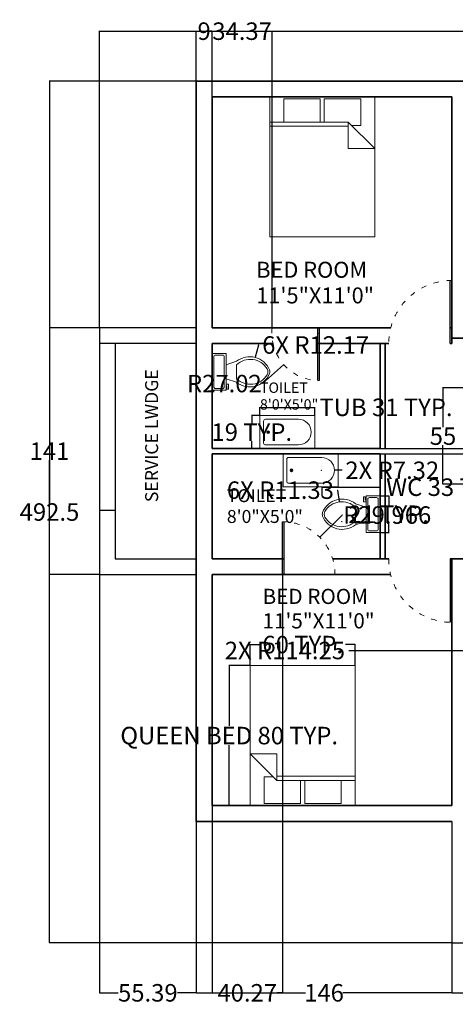
# Model space of a CAD drawing. Units: inches. Extents: x 37 to 687, y -399 to 163.
# Tile 1 of 4: x 37 to 286, y -399 to 163. Entities that reach past the tile are written whole.
import ezdxf

# ---------------------------------------------------------------- set-up
doc = ezdxf.new("R2010")
doc.units = ezdxf.units.IN
doc.header["$MEASUREMENT"] = 0
doc.linetypes.add('ACAD_ISO03W100', pattern=[30, 12, -18])
for name, color, linetype, lineweight in [('A-ANNO-DIMS', 2, 'Continuous', 18), ('A-AREA-IDEN', 7, 'Continuous', 18), ('A-DOOR', 4, 'Continuous', 25), ('A-DOOR-SWNG', 4, 'ACAD_ISO03W100', 13), ('A-FLOR-FIXT', 9, 'Continuous', 18), ('A-FLOR-OTLN', 7, 'Continuous', 25), ('A-FURN', 8, 'Continuous', 18), ('A-WALL', 7, 'Continuous', 35), ('A-WALL-OVHD', 7, 'ACAD_ISO03W100', 18)]:
    doc.layers.add(name, color=color, linetype=linetype, lineweight=lineweight)
doc.styles.get("Standard").update_dxf_attribs({"font": 'arial.ttf'})
doc.dimstyles.get("Standard").update_dxf_attribs({"dimtxt": 10, "dimasz": 0.18, "dimexe": 0.18, "dimexo": 0.0625, "dimgap": 0.09, "dimtad": 0, "dimtih": 1, "dimtoh": 1, "dimdec": 0, "dimzin": 0, "dimdsep": 46, "dimlunit": 3, "dimtxsty": 'Standard', "dimcen": 0.09, "dimadec": 0, "dimazin": 0, "dimtfac": 1, "dimtdec": 0, "dimtofl": 0, "dimtmove": 0, "dimatfit": 3, "dimfxl": 1, "dimtolj": 1, "dimtzin": 0, "dimarcsym": 0})

# ---------------------------------------------------------------- blocks, each defined once
blk = doc.blocks.new('Bed - Queen')
for p, q in [((0, -80.00003), (0, 0)), ((0, 0), (59.99999, 0)), ((59.99999, 0), (59.99999, -80.00003)), ((7.99999, -1.2), (28.79998, -1.2)), ((7.99999, -14.4), (7.99999, -1.2)), ((28.79998, -1.2), (28.79998, -14.4)), ((31.19999, -1.2), (51.99999, -1.2)), ((31.19999, -14.4), (31.19999, -1.2)), ((51.99999, -1.2), (51.99999, -16.4)), ((0, -14.4), (44.8, -14.4)), ((44.8, -16.8), (0, -16.8)), ((59.99999, -29.6), (44.8, -14.4)), ((44.8, -14.4), (44.8, -29.6)), ((51.99999, -16.4), (46.79936, -16.4)), ((44.8, -29.6), (59.99999, -29.6)), ((59.99999, -80.00003), (0, -80.00003))]:
    blk.add_line(p, q)
blk = doc.blocks.new('Toilet - top')
for p, q in [((9.5, -6), (9.5, -2)), ((-10, -8.5), (-8, -8.5)), ((-10, -9.5), (-10, -8.5)), ((-7, -9.5), (-10, -9.5)), ((-8, -8.5), (-8, -8)), ((-7, -8), (-7, -9.5)), ((-4, -8), (-6, -14)), ((4, -8), (6, -14)), ((4, -14), (-4, -14))]:
    blk.add_line(p, q)
blk.add_lwpolyline([(10.5, -8), (10.5, 0), (-10.5, 0), (-10.5, -8)], close=True)
for points in [[(-9.5, -2), (-9.5, -6)], [(8.5, -1), (-8.5, -1)], [(-8.5, -7), (8.5, -7)]]:
    blk.add_lwpolyline(points)
for centre, radius, start, end in [((-8.62, -1.88), 0.884, 81.8699, 188.1301), ((8.62, -1.88), 0.884, 351.8699, 98.1301), ((-8.62, -6.12), 0.884, 171.8699, 278.1301), ((8.62, -6.12), 0.884, 261.8699, 8.1301), ((3.52, -21.58), 12.17, 141.4691, 247.9714), ((4.2, -21.82), 11.33, 136.3677, 238.9468), ((-3.52, -21.58), 12.17, 292.0284, 38.5307), ((-4.2, -21.82), 11.33, 301.053, 43.6321), ((0, -27.88), 4, 245.7318, 294.2682), ((0, -29), 4, 254.8605, 285.1395)]:
    blk.add_arc(centre, radius, start, end)
blk = doc.blocks.new('Bath Tub - 26 x 60 in.')
for p, q in [((8, -18), (10, -18)), ((9, -17), (9, -19))]:
    blk.add_line(p, q)
blk.add_lwpolyline([(0, -36), (0, 0), (60, 0), (60, -36)], close=True)
for points in [[(4, -30), (4, -6)], [(6, -4), (42, -4)], [(42, -32), (6, -32)]]:
    blk.add_lwpolyline(points)
for radius in [1.5, 1]:
    blk.add_circle((9, -18), radius)
for centre, radius, start, end in [((5.75, -5.75), 1.77, 81.8699, 188.1301), ((42, -18), 14, 270, 90), ((5.75, -30.25), 1.77, 171.8699, 278.1301)]:
    blk.add_arc(centre, radius, start, end)
blk = doc.blocks.new('*D9')
at = {"layer": 'A-ANNO-DIMS', "color": 0, "lineweight": -2, "ltscale": 0.25, "transparency": 16777216}
for p, q in [((168.43, -205.68), (156.31, -205.68)), ((156.49, -205.86), (156.49, -240.12)), ((156.49, -285.5), (156.49, -251.25)), ((168.43, -285.68), (156.31, -285.68))]:
    blk.add_line(p, q, dxfattribs=at)
at = {"layer": 'A-ANNO-DIMS', "color": 0, "ltscale": 0.25, "transparency": 16777216}
for points in [[(156.46, -205.86), (156.52, -205.86), (156.49, -205.68)], [(156.46, -285.5), (156.52, -285.5), (156.49, -285.68)]]:
    blk.add_solid(points, dxfattribs=at)
at = {"layer": 'Defpoints', "color": 0, "ltscale": 0.25, "transparency": 16777216}
for p in [(168.49, -205.68), (156.49, -285.68), (168.49, -285.68)]:
    blk.add_point(p, dxfattribs=at)
at = {"layer": 'A-ANNO-DIMS', "color": 0, "ltscale": 0.25, "transparency": 16777216, "insert": (156.49, -245.68), "char_height": 10, "attachment_point": 5}
blk.add_mtext('\\A1;QUEEN BED 80 TYP.', dxfattribs=at)
blk = doc.blocks.new('*D10')
at = {"layer": 'A-ANNO-DIMS', "color": 0, "lineweight": -2, "ltscale": 0.25, "transparency": 16777216}
for p, q in [((168.49, -205.62), (168.49, -193.5)), ((168.67, -193.68), (174.04, -193.68)), ((228.31, -193.68), (222.95, -193.68)), ((228.49, -205.62), (228.49, -193.5))]:
    blk.add_line(p, q, dxfattribs=at)
at = {"layer": 'A-ANNO-DIMS', "color": 0, "ltscale": 0.25, "transparency": 16777216}
for points in [[(168.67, -193.65), (168.67, -193.71), (168.49, -193.68)], [(228.31, -193.65), (228.31, -193.71), (228.49, -193.68)]]:
    blk.add_solid(points, dxfattribs=at)
at = {"layer": 'Defpoints', "color": 0, "ltscale": 0.25, "transparency": 16777216}
for p in [(168.49, -193.68), (168.49, -205.68), (228.49, -205.68)]:
    blk.add_point(p, dxfattribs=at)
at = {"layer": 'A-ANNO-DIMS', "color": 0, "ltscale": 0.25, "transparency": 16777216, "insert": (198.49, -193.68), "char_height": 10, "attachment_point": 5}
blk.add_mtext('\\A1;60 TYP.', dxfattribs=at)
blk = doc.blocks.new('*D15')
at = {"layer": 'A-ANNO-DIMS', "color": 0, "lineweight": -2, "ltscale": 0.25, "transparency": 16777216}
for p, q in [((174.08, -62.8), (174.08, -57.97)), ((174.26, -58.15), (205.27, -58.15)), ((205.45, -62.8), (205.45, -57.97)), ((205.45, -58.15), (205.63, -58.15))]:
    blk.add_line(p, q, dxfattribs=at)
at = {"layer": 'A-ANNO-DIMS', "color": 0, "ltscale": 0.25, "transparency": 16777216}
for points in [[(174.26, -58.12), (174.26, -58.18), (174.08, -58.15)], [(205.27, -58.12), (205.27, -58.18), (205.45, -58.15)]]:
    blk.add_solid(points, dxfattribs=at)
at = {"layer": 'Defpoints', "color": 0, "ltscale": 0.25, "transparency": 16777216}
for p in [(205.45, -58.15), (174.08, -62.86), (205.45, -62.86)]:
    blk.add_point(p, dxfattribs=at)
at = {"layer": 'A-ANNO-DIMS', "color": 0, "ltscale": 0.25, "transparency": 16777216, "insert": (246.1, -58.15), "char_height": 10, "attachment_point": 5}
blk.add_mtext('\\A1;TUB 31 TYP.', dxfattribs=at)
blk = doc.blocks.new('*D16')
at = {"layer": 'A-ANNO-DIMS', "color": 0, "lineweight": -2, "ltscale": 0.25, "transparency": 16777216}
for p, q in [((174.02, -62.86), (169.2, -62.86)), ((169.38, -63.04), (169.38, -67.08)), ((169.38, -81.5), (169.38, -77.47)), ((174.02, -81.68), (169.2, -81.68))]:
    blk.add_line(p, q, dxfattribs=at)
at = {"layer": 'A-ANNO-DIMS', "color": 0, "ltscale": 0.25, "transparency": 16777216}
for points in [[(169.35, -63.04), (169.41, -63.04), (169.38, -62.86)], [(169.35, -81.5), (169.41, -81.5), (169.38, -81.68)]]:
    blk.add_solid(points, dxfattribs=at)
at = {"layer": 'Defpoints', "color": 0, "ltscale": 0.25, "transparency": 16777216}
for p in [(169.38, -62.86), (174.08, -62.86), (174.08, -81.68)]:
    blk.add_point(p, dxfattribs=at)
at = {"layer": 'A-ANNO-DIMS', "color": 0, "ltscale": 0.25, "transparency": 16777216, "insert": (169.38, -72.27), "char_height": 10, "attachment_point": 5}
blk.add_mtext('\\A1;19 TYP.', dxfattribs=at)
blk = doc.blocks.new('*D17')
at = {"layer": 'A-ANNO-DIMS', "color": 0, "lineweight": -2, "ltscale": 0.25, "transparency": 16777216}
for p, q in [((209.64, -108.64), (209.64, -103.57)), ((209.82, -103.75), (242.51, -103.75)), ((242.69, -108.64), (242.69, -103.57)), ((242.69, -103.75), (242.87, -103.75))]:
    blk.add_line(p, q, dxfattribs=at)
at = {"layer": 'A-ANNO-DIMS', "color": 0, "ltscale": 0.25, "transparency": 16777216}
for points in [[(209.82, -103.72), (209.82, -103.78), (209.64, -103.75)], [(242.51, -103.72), (242.51, -103.78), (242.69, -103.75)]]:
    blk.add_solid(points, dxfattribs=at)
at = {"layer": 'Defpoints', "color": 0, "ltscale": 0.25, "transparency": 16777216}
for p in [(242.69, -103.75), (209.64, -108.71), (242.69, -108.71)]:
    blk.add_point(p, dxfattribs=at)
at = {"layer": 'A-ANNO-DIMS', "color": 0, "ltscale": 0.25, "transparency": 16777216, "insert": (281.08, -103.75), "char_height": 10, "attachment_point": 5}
blk.add_mtext('\\A1;WC 33 TYP.', dxfattribs=at)
blk = doc.blocks.new('*D18')
at = {"layer": 'A-ANNO-DIMS', "color": 0, "lineweight": -2, "ltscale": 0.25, "transparency": 16777216}
for p, q in [((242.75, -108.71), (247.82, -108.71)), ((247.64, -108.89), (247.64, -114.09)), ((247.64, -129.53), (247.64, -124.32)), ((242.75, -129.71), (247.82, -129.71))]:
    blk.add_line(p, q, dxfattribs=at)
at = {"layer": 'A-ANNO-DIMS', "color": 0, "ltscale": 0.25, "transparency": 16777216}
for points in [[(247.61, -108.89), (247.67, -108.89), (247.64, -108.71)], [(247.61, -129.53), (247.67, -129.53), (247.64, -129.71)]]:
    blk.add_solid(points, dxfattribs=at)
at = {"layer": 'Defpoints', "color": 0, "ltscale": 0.25, "transparency": 16777216}
for p in [(242.69, -108.71), (242.69, -129.71), (247.64, -129.71)]:
    blk.add_point(p, dxfattribs=at)
at = {"layer": 'A-ANNO-DIMS', "color": 0, "ltscale": 0.25, "transparency": 16777216, "insert": (247.64, -119.21), "char_height": 10, "attachment_point": 5}
blk.add_mtext('\\A1;21 TYP.', dxfattribs=at)
blk = doc.blocks.new('*D22')
at = {"layer": 'A-ANNO-DIMS', "color": 0, "lineweight": -2, "ltscale": 0.25, "transparency": 16777216}
for p, q in [((292.25, -47.07), (278.48, -47.07)), ((278.66, -47.25), (278.66, -69.4)), ((278.66, -101.89), (278.66, -79.75)), ((292.25, -102.07), (278.48, -102.07))]:
    blk.add_line(p, q, dxfattribs=at)
at = {"layer": 'A-ANNO-DIMS', "color": 0, "ltscale": 0.25, "transparency": 16777216}
for points in [[(278.63, -47.25), (278.69, -47.25), (278.66, -47.07)], [(278.63, -101.89), (278.69, -101.89), (278.66, -102.07)]]:
    blk.add_solid(points, dxfattribs=at)
at = {"layer": 'Defpoints', "color": 0, "ltscale": 0.25, "transparency": 16777216}
for p in [(278.66, -47.07), (292.31, -47.07), (292.31, -102.07)]:
    blk.add_point(p, dxfattribs=at)
at = {"layer": 'A-ANNO-DIMS', "color": 0, "ltscale": 0.25, "transparency": 16777216, "insert": (278.66, -74.57), "char_height": 10, "attachment_point": 5}
blk.add_mtext('\\A1;55', dxfattribs=at)
blk = doc.blocks.new('*D27')
at = {"layer": 'A-ANNO-DIMS', "color": 0, "lineweight": -2, "ltscale": 0.25, "transparency": 16777216}
for p, q in [((82.29, -12.62), (82.29, 157)), ((82.47, 156.82), (344.98, 156.82)), ((641.3, 156.82), (378.8, 156.82)), ((641.48, 53.47), (641.48, 157))]:
    blk.add_line(p, q, dxfattribs=at)
at = {"layer": 'A-ANNO-DIMS', "color": 0, "ltscale": 0.25, "transparency": 16777216}
for points in [[(82.47, 156.85), (82.47, 156.79), (82.29, 156.82)], [(641.3, 156.85), (641.3, 156.79), (641.48, 156.82)]]:
    blk.add_solid(points, dxfattribs=at)
at = {"layer": 'Defpoints', "color": 0, "ltscale": 0.25, "transparency": 16777216}
for p in [(641.48, 156.82), (641.48, 53.4), (82.29, -12.68)]:
    blk.add_point(p, dxfattribs=at)
at = {"layer": 'A-ANNO-DIMS', "color": 0, "ltscale": 0.25, "transparency": 16777216, "insert": (361.89, 156.82), "char_height": 10, "attachment_point": 5}
blk.add_mtext('\\A1;559.2', dxfattribs=at)
blk = doc.blocks.new('*D28')
at = {"layer": 'A-ANNO-DIMS', "color": 0, "lineweight": -2, "ltscale": 0.25, "transparency": 16777216}
for p, q in [((137.62, 128.32), (53.61, 128.32)), ((53.79, 128.14), (53.79, -112.73)), ((53.79, -363.99), (53.79, -123.12)), ((283.62, -364.17), (53.61, -364.17))]:
    blk.add_line(p, q, dxfattribs=at)
at = {"layer": 'A-ANNO-DIMS', "color": 0, "ltscale": 0.25, "transparency": 16777216}
for points in [[(53.76, 128.14), (53.82, 128.14), (53.79, 128.32)], [(53.76, -363.99), (53.82, -363.99), (53.79, -364.17)]]:
    blk.add_solid(points, dxfattribs=at)
at = {"layer": 'Defpoints', "color": 0, "ltscale": 0.25, "transparency": 16777216}
for p in [(137.69, 128.32), (53.79, -364.17), (283.69, -364.17)]:
    blk.add_point(p, dxfattribs=at)
at = {"layer": 'A-ANNO-DIMS', "color": 0, "ltscale": 0.25, "transparency": 16777216, "insert": (53.79, -117.93), "char_height": 10, "attachment_point": 5}
blk.add_mtext('\\A1;492.5', dxfattribs=at)
blk = doc.blocks.new('*D29')
at = {"layer": 'A-ANNO-DIMS', "color": 0, "lineweight": -2, "ltscale": 0.25, "transparency": 16777216}
for p, q in [((82.29, -153.75), (82.29, -392.85)), ((137.69, -294.75), (137.69, -392.85)), ((82.47, -392.67), (93.02, -392.67)), ((137.51, -392.67), (126.96, -392.67))]:
    blk.add_line(p, q, dxfattribs=at)
at = {"layer": 'A-ANNO-DIMS', "color": 0, "ltscale": 0.25, "transparency": 16777216}
for points in [[(82.47, -392.64), (82.47, -392.7), (82.29, -392.67)], [(137.51, -392.64), (137.51, -392.7), (137.69, -392.67)]]:
    blk.add_solid(points, dxfattribs=at)
at = {"layer": 'Defpoints', "color": 0, "ltscale": 0.25, "transparency": 16777216}
for p in [(82.29, -153.68), (137.69, -294.68), (137.69, -392.67)]:
    blk.add_point(p, dxfattribs=at)
at = {"layer": 'A-ANNO-DIMS', "color": 0, "ltscale": 0.25, "transparency": 16777216, "insert": (109.99, -392.67), "char_height": 10, "attachment_point": 5}
blk.add_mtext('\\A1;55.39', dxfattribs=at)
blk = doc.blocks.new('*D30')
at = {"layer": 'A-ANNO-DIMS', "color": 0, "lineweight": -2, "ltscale": 0.25, "transparency": 16777216}
for p, q in [((137.69, -294.75), (137.69, -392.85)), ((283.69, -294.75), (283.69, -392.85)), ((137.87, -392.67), (200.02, -392.67)), ((283.51, -392.67), (221.35, -392.67))]:
    blk.add_line(p, q, dxfattribs=at)
at = {"layer": 'A-ANNO-DIMS', "color": 0, "ltscale": 0.25, "transparency": 16777216}
for points in [[(137.87, -392.64), (137.87, -392.7), (137.69, -392.67)], [(283.51, -392.64), (283.51, -392.7), (283.69, -392.67)]]:
    blk.add_solid(points, dxfattribs=at)
at = {"layer": 'Defpoints', "color": 0, "ltscale": 0.25, "transparency": 16777216}
for p in [(137.69, -294.68), (283.69, -294.68), (283.69, -392.67)]:
    blk.add_point(p, dxfattribs=at)
at = {"layer": 'A-ANNO-DIMS', "color": 0, "ltscale": 0.25, "transparency": 16777216, "insert": (210.69, -392.67), "char_height": 10, "attachment_point": 5}
blk.add_mtext('\\A1;146', dxfattribs=at)
blk = doc.blocks.new('*D31')
at = {"layer": 'A-ANNO-DIMS', "color": 0, "lineweight": -2, "ltscale": 0.25, "transparency": 16777216}
for p, q in [((283.69, -364.23), (283.69, -392.85)), ((444.69, -364.23), (444.69, -392.85)), ((283.87, -392.67), (354.48, -392.67)), ((444.51, -392.67), (373.89, -392.67))]:
    blk.add_line(p, q, dxfattribs=at)
at = {"layer": 'A-ANNO-DIMS', "color": 0, "ltscale": 0.25, "transparency": 16777216}
for points in [[(283.87, -392.64), (283.87, -392.7), (283.69, -392.67)], [(444.51, -392.64), (444.51, -392.7), (444.69, -392.67)]]:
    blk.add_solid(points, dxfattribs=at)
at = {"layer": 'Defpoints', "color": 0, "ltscale": 0.25, "transparency": 16777216}
for p in [(283.69, -364.17), (444.69, -364.17), (444.69, -392.67)]:
    blk.add_point(p, dxfattribs=at)
at = {"layer": 'A-ANNO-DIMS', "color": 0, "ltscale": 0.25, "transparency": 16777216, "insert": (364.19, -392.67), "char_height": 10, "attachment_point": 5}
blk.add_mtext('\\A1;161', dxfattribs=at)
blk = doc.blocks.new('*D40')
at = {"layer": 'A-ANNO-DIMS', "color": 0, "lineweight": -2, "ltscale": 0.25, "transparency": 16777216}
for p, q in [((82.23, -12.68), (53.61, -12.68)), ((53.79, -12.86), (53.79, -78.07)), ((53.79, -153.5), (53.79, -88.3)), ((82.23, -153.68), (53.61, -153.68))]:
    blk.add_line(p, q, dxfattribs=at)
at = {"layer": 'A-ANNO-DIMS', "color": 0, "ltscale": 0.25, "transparency": 16777216}
for points in [[(53.76, -12.86), (53.82, -12.86), (53.79, -12.68)], [(53.76, -153.5), (53.82, -153.5), (53.79, -153.68)]]:
    blk.add_solid(points, dxfattribs=at)
at = {"layer": 'Defpoints', "color": 0, "ltscale": 0.25, "transparency": 16777216}
for p in [(53.79, -12.68), (82.29, -12.68), (82.29, -153.68)]:
    blk.add_point(p, dxfattribs=at)
at = {"layer": 'A-ANNO-DIMS', "color": 0, "ltscale": 0.25, "transparency": 16777216, "insert": (53.79, -83.18), "char_height": 10, "attachment_point": 5}
blk.add_mtext('\\A1;141', dxfattribs=at)
blk = doc.blocks.new('*D41')
at = {"layer": 'A-ANNO-DIMS', "color": 0, "lineweight": -2, "ltscale": 0.25, "transparency": 16777216}
for p, q in [((137.69, -12.62), (137.69, 157)), ((137.87, 156.82), (138.81, 156.82)), ((146.51, 156.82), (145.56, 156.82)), ((146.69, -12.62), (146.69, 157))]:
    blk.add_line(p, q, dxfattribs=at)
at = {"layer": 'A-ANNO-DIMS', "color": 0, "ltscale": 0.25, "transparency": 16777216}
for points in [[(137.87, 156.85), (137.87, 156.79), (137.69, 156.82)], [(146.51, 156.85), (146.51, 156.79), (146.69, 156.82)]]:
    blk.add_solid(points, dxfattribs=at)
at = {"layer": 'Defpoints', "color": 0, "ltscale": 0.25, "transparency": 16777216}
for p in [(146.69, 156.82), (137.69, -12.68), (146.69, -12.68)]:
    blk.add_point(p, dxfattribs=at)
at = {"layer": 'A-ANNO-DIMS', "color": 0, "ltscale": 0.25, "transparency": 16777216, "insert": (142.19, 156.82), "char_height": 10, "attachment_point": 5}
blk.add_mtext('\\A1;9', dxfattribs=at)
blk = doc.blocks.new('*D42')
at = {"layer": 'A-ANNO-DIMS', "color": 0, "lineweight": -2, "ltscale": 0.25, "transparency": 16777216}
for p, q in [((146.505166, 156.815421), (146.325166, 156.815421)), ((146.685166, -12.622079), (146.685166, 156.995421)), ((181.054232, -12.622079), (181.054232, 156.995421)), ((181.234232, 156.815421), (181.414232, 156.815421))]:
    blk.add_line(p, q, dxfattribs=at)
at = {"layer": 'A-ANNO-DIMS', "color": 0, "ltscale": 0.25, "transparency": 16777216}
for points in [[(146.505166, 156.845421), (146.505166, 156.785421), (146.685166, 156.815421)], [(181.234232, 156.845421), (181.234232, 156.785421), (181.054232, 156.815421)]]:
    blk.add_solid(points, dxfattribs=at)
at = {"layer": 'Defpoints', "color": 0, "ltscale": 0.25, "transparency": 16777216}
for p in [(181.054232, 156.815421), (146.685166, -12.684579), (181.054232, -12.684579)]:
    blk.add_point(p, dxfattribs=at)
at = {"layer": 'A-ANNO-DIMS', "color": 0, "ltscale": 0.25, "transparency": 16777216, "insert": (163.869699, 156.815421), "char_height": 10, "attachment_point": 5}
blk.add_mtext('\\A1;34.37', dxfattribs=at)
blk = doc.blocks.new('*D43')
at = {"layer": 'A-ANNO-DIMS', "color": 0, "lineweight": -2, "ltscale": 0.25, "transparency": 16777216}
for p, q in [((146.69, -153.75), (146.69, -392.85)), ((186.95, -153.75), (186.95, -392.85)), ((146.87, -392.67), (149.65, -392.67)), ((186.77, -392.67), (183.98, -392.67))]:
    blk.add_line(p, q, dxfattribs=at)
at = {"layer": 'A-ANNO-DIMS', "color": 0, "ltscale": 0.25, "transparency": 16777216}
for points in [[(146.87, -392.64), (146.87, -392.7), (146.69, -392.67)], [(186.77, -392.64), (186.77, -392.7), (186.95, -392.67)]]:
    blk.add_solid(points, dxfattribs=at)
at = {"layer": 'Defpoints', "color": 0, "ltscale": 0.25, "transparency": 16777216}
for p in [(146.69, -153.68), (186.95, -153.68), (186.95, -392.67)]:
    blk.add_point(p, dxfattribs=at)
at = {"layer": 'A-ANNO-DIMS', "color": 0, "ltscale": 0.25, "transparency": 16777216, "insert": (166.82, -392.67), "char_height": 10, "attachment_point": 5}
blk.add_mtext('\\A1;40.27', dxfattribs=at)
blk = doc.blocks.new('*D44')
at = {"layer": 'A-ANNO-DIMS', "color": 0, "lineweight": -2, "ltscale": 0.25, "transparency": 16777216}
for p, q in [((242.75, -81.68), (670.18, -81.68)), ((670, -81.68), (670, -81.5)), ((670, -81.5), (670.18, -81.5)), ((670, -84.5), (670, -81.86)), ((242.75, -84.68), (670.18, -84.68))]:
    blk.add_line(p, q, dxfattribs=at)
at = {"layer": 'A-ANNO-DIMS', "color": 0, "ltscale": 0.25, "transparency": 16777216}
for points in [[(669.97, -81.86), (670.03, -81.86), (670, -81.68)], [(669.97, -84.5), (670.03, -84.5), (670, -84.68)]]:
    blk.add_solid(points, dxfattribs=at)
at = {"layer": 'Defpoints', "color": 0, "ltscale": 0.25, "transparency": 16777216}
for p in [(242.69, -81.68), (670, -81.68), (242.69, -84.68)]:
    blk.add_point(p, dxfattribs=at)
at = {"layer": 'A-ANNO-DIMS', "color": 0, "ltscale": 0.25, "transparency": 16777216, "insert": (673.54, -81.5), "char_height": 10, "attachment_point": 5}
blk.add_mtext('\\A1;3', dxfattribs=at)
blk = doc.blocks.new('*D51')
at = {"layer": 'A-ANNO-DIMS', "color": 0, "lineweight": -2, "ltscale": 0.25, "transparency": 16777216}
for p, q in [((220.99, -119.68), (208.35, -132.22)), ((221.17, -119.68), (220.99, -119.68)), ((186.86, -153.45), (187.04, -153.45)), ((186.95, -153.54), (186.95, -153.36))]:
    blk.add_line(p, q, dxfattribs=at)
at = {"layer": 'A-ANNO-DIMS', "color": 0, "ltscale": 0.25, "transparency": 16777216}
blk.add_solid([(208.33, -132.19), (208.37, -132.24), (208.22, -132.34)], dxfattribs=at)
at = {"layer": 'Defpoints', "color": 0, "ltscale": 0.25, "transparency": 16777216}
for p in [(208.22, -132.34), (186.95, -153.45)]:
    blk.add_point(p, dxfattribs=at)
at = {"layer": 'A-ANNO-DIMS', "color": 0, "ltscale": 0.25, "transparency": 16777216, "insert": (246.8, -119.68), "char_height": 10, "attachment_point": 5}
blk.add_mtext('\\A1;R29.966', dxfattribs=at)
blk = doc.blocks.new('*D52')
at = {"layer": 'A-ANNO-DIMS', "color": 0, "lineweight": -2, "ltscale": 0.25, "transparency": 16777216}
for p, q in [((207.8, -15.8), (207.98, -15.8)), ((207.89, -15.89), (207.89, -15.71)), ((175.61, -44.55), (187.58, -33.89)), ((175.43, -44.55), (175.61, -44.55))]:
    blk.add_line(p, q, dxfattribs=at)
at = {"layer": 'A-ANNO-DIMS', "color": 0, "ltscale": 0.25, "transparency": 16777216}
blk.add_solid([(187.56, -33.87), (187.6, -33.92), (187.71, -33.77)], dxfattribs=at)
at = {"layer": 'Defpoints', "color": 0, "ltscale": 0.25, "transparency": 16777216}
for p in [(207.89, -15.8), (187.71, -33.77)]:
    blk.add_point(p, dxfattribs=at)
at = {"layer": 'A-ANNO-DIMS', "color": 0, "ltscale": 0.25, "transparency": 16777216, "insert": (153.73, -44.55), "char_height": 10, "attachment_point": 5}
blk.add_mtext('\\A1;R27.02', dxfattribs=at)
blk = doc.blocks.new('*D55')
at = {"layer": 'A-ANNO-DIMS', "color": 0, "lineweight": -2, "ltscale": 0.25, "transparency": 16777216}
for p, q in [((224.82, -197.06), (293.19, -197.06)), ((407.53, -197.06), (407.71, -197.06)), ((407.62, -197.15), (407.62, -196.97))]:
    blk.add_line(p, q, dxfattribs=at)
at = {"layer": 'A-ANNO-DIMS', "color": 0, "ltscale": 0.25, "transparency": 16777216}
blk.add_solid([(293.19, -197.03), (293.19, -197.09), (293.37, -197.06)], dxfattribs=at)
at = {"layer": 'Defpoints', "color": 0, "ltscale": 0.25, "transparency": 16777216}
for p in [(293.37, -197.06), (407.62, -197.06)]:
    blk.add_point(p, dxfattribs=at)
at = {"layer": 'A-ANNO-DIMS', "color": 0, "ltscale": 0.25, "transparency": 16777216, "insert": (188.33, -197.06), "char_height": 10, "attachment_point": 5}
blk.add_mtext('\\A1;2X R114.25', dxfattribs=at)
blk = doc.blocks.new('*D58')
at = {"layer": 'A-ANNO-DIMS', "color": 0, "lineweight": -2, "ltscale": 0.25, "transparency": 16777216}
for p, q in [((173.21, -22.51), (171.4, -29.4)), ((173.39, -22.51), (173.21, -22.51)), ((168.18, -41.34), (168.36, -41.34)), ((168.27, -41.43), (168.27, -41.25))]:
    blk.add_line(p, q, dxfattribs=at)
at = {"layer": 'A-ANNO-DIMS', "color": 0, "ltscale": 0.25, "transparency": 16777216}
blk.add_solid([(171.37, -29.39), (171.43, -29.41), (171.36, -29.57)], dxfattribs=at)
at = {"layer": 'Defpoints', "color": 0, "ltscale": 0.25, "transparency": 16777216}
for p in [(171.36, -29.57), (168.27, -41.34)]:
    blk.add_point(p, dxfattribs=at)
at = {"layer": 'A-ANNO-DIMS', "color": 0, "ltscale": 0.25, "transparency": 16777216, "insert": (205.91, -22.51), "char_height": 10, "attachment_point": 5}
blk.add_mtext('\\A1;6X R12.17', dxfattribs=at)
blk = doc.blocks.new('*D59')
at = {"layer": 'A-ANNO-DIMS', "color": 0, "lineweight": -2, "ltscale": 0.25, "transparency": 16777216}
for p, q in [((218.27, -105.44), (218.45, -105.44)), ((218.45, -105.44), (219.33, -112)), ((220.78, -123.41), (220.96, -123.41)), ((220.87, -123.5), (220.87, -123.32))]:
    blk.add_line(p, q, dxfattribs=at)
at = {"layer": 'A-ANNO-DIMS', "color": 0, "ltscale": 0.25, "transparency": 16777216}
blk.add_solid([(219.36, -112), (219.3, -112), (219.36, -112.18)], dxfattribs=at)
at = {"layer": 'Defpoints', "color": 0, "ltscale": 0.25, "transparency": 16777216}
for p in [(219.36, -112.18), (220.87, -123.41)]:
    blk.add_point(p, dxfattribs=at)
at = {"layer": 'A-ANNO-DIMS', "color": 0, "ltscale": 0.25, "transparency": 16777216, "insert": (185.75, -105.44), "char_height": 10, "attachment_point": 5}
blk.add_mtext('\\A1;6X R11.33', dxfattribs=at)
blk = doc.blocks.new('*D60')
at = {"layer": 'A-ANNO-DIMS', "color": 0, "lineweight": -2, "ltscale": 0.25, "transparency": 16777216}
for p, q in [((209.24, -94.1), (209.42, -94.1)), ((209.33, -94.19), (209.33, -94.01)), ((221.04, -94.1), (216.83, -94.1))]:
    blk.add_line(p, q, dxfattribs=at)
at = {"layer": 'A-ANNO-DIMS', "color": 0, "ltscale": 0.25, "transparency": 16777216}
blk.add_solid([(216.83, -94.07), (216.83, -94.13), (216.65, -94.1)], dxfattribs=at)
at = {"layer": 'Defpoints', "color": 0, "ltscale": 0.25, "transparency": 16777216}
for p in [(209.33, -94.1), (216.65, -94.1)]:
    blk.add_point(p, dxfattribs=at)
at = {"layer": 'A-ANNO-DIMS', "color": 0, "ltscale": 0.25, "transparency": 16777216, "insert": (249.68, -94.1), "char_height": 10, "attachment_point": 5}
blk.add_mtext('\\A1;2X R7.32', dxfattribs=at)

msp = doc.modelspace()

# ---------------------------------------------------------------- linework, layer by layer
at = {"layer": 'A-DOOR'}
for p, q in [((282.6852, -21.6846), (282.6852, 14.3724)), ((283.6852, -21.6846), (283.6852, 14.3724)), ((207.8937, -12.6846), (177.9197, -12.6846)), ((177.9197, -12.6846), (181.0542, -12.6846)), ((206.8937, -12.6846), (206.8937, -42.824)), ((207.8937, -12.6846), (207.8937, -42.824)), ((283.6852, -21.6846), (282.6852, -21.6846))]:
    msp.add_line(p, q, dxfattribs=at)
at = {"layer": 'A-DOOR', "ltscale": 0.25}
for p, q in [((186.9515, -153.6846), (186.9515, -123.4817)), ((187.9515, -153.6846), (187.9515, -123.4817)), ((283.6852, -144.6846), (282.6852, -144.6846)), ((282.6852, -144.6846), (282.6852, -180.9603)), ((283.6852, -144.6846), (283.6852, -180.9603)), ((186.9515, -153.6846), (216.9162, -153.6846))]:
    msp.add_line(p, q, dxfattribs=at)
at = {"layer": 'A-DOOR-SWNG', "ltscale": 0.25}
for centre, radius, start, end in [((283.6852, -21.6277), 36, 90, 180.09058), ((207.8937, -15.8039), 27.0201, 173.370656, 270), ((186.9515, -153.4474), 29.9657, 359.546558, 90), ((283.6852, -144.9592), 36.001, 179.562888, 270)]:
    msp.add_arc(centre, radius, start, end, dxfattribs=at)
at = {"layer": 'A-FLOR-OTLN', "ltscale": 0.25}
for p, q in [((137.6852, -12.6846), (82.2949, -12.6846)), ((82.2949, -12.6846), (82.2949, -153.6846)), ((137.6852, -21.6846), (82.2949, -21.6846)), ((91.2949, -21.6846), (91.2949, -144.6846)), ((91.2949, -117.1166), (82.2949, -117.1166)), ((91.2949, -144.6846), (137.6852, -144.6846)), ((82.2949, -153.6846), (137.6852, -153.6846))]:
    msp.add_line(p, q, dxfattribs=at)
at = {"layer": 'A-FLOR-OTLN'}
for p, q in [((283.6852, -294.6846), (283.6852, -364.1681)), ((283.6852, -364.1681), (444.6852, -364.1681))]:
    msp.add_line(p, q, dxfattribs=at)
at = {"layer": 'A-WALL'}
for p, q in [((137.6852, 128.3154), (595.6852, 128.3154)), ((137.6852, 128.3154), (137.6852, -294.6846)), ((137.6852, 119.3154), (137.6852, -12.6846)), ((146.6852, 119.3154), (146.6852, -12.6846)), ((146.6852, 119.3154), (283.6852, 119.3154)), ((283.6852, 119.3154), (283.6852, -21.6846)), ((248.8136, -12.6846), (146.6852, -12.6846)), ((283.6852, -12.6846), (282.6852, -12.6846)), ((137.6852, -21.6846), (137.6852, -81.6846)), ((146.6852, -21.6846), (146.6852, -81.6846)), ((181.5213, -21.6846), (146.6852, -21.6846)), ((247.6852, -21.6846), (206.8937, -21.6846)), ((242.6852, -81.6846), (242.6852, -21.6846)), ((245.6852, -81.6846), (245.6852, -21.6846)), ((283.6852, -21.6846), (282.6852, -21.6846)), ((146.6852, -81.6846), (242.6852, -81.6846)), ((137.6852, -84.6846), (137.6852, -144.6846)), ((146.6852, -84.6846), (242.6852, -84.6846)), ((146.6852, -84.6846), (146.6852, -144.6846)), ((242.6852, -144.6846), (242.6852, -84.6846)), ((245.6852, -144.6846), (245.6852, -84.6846)), ((146.6852, -144.6846), (187.9515, -144.6846)), ((215.6073, -144.6846), (242.6852, -144.6846)), ((247.6852, -144.6846), (242.6852, -144.6846)), ((290.6852, -144.6846), (282.6852, -144.6846)), ((283.6852, -285.6846), (283.6852, -144.6846)), ((146.6852, -153.6846), (242.6852, -153.6846)), ((146.6852, -153.6846), (146.6852, -285.6846)), ((248.7575, -153.6846), (242.6852, -153.6846)), ((283.6852, -153.6846), (282.6852, -153.6846)), ((283.6852, -259.1681), (283.6852, -285.6846)), ((146.6852, -285.6846), (283.6852, -285.6846)), ((137.6852, -294.6846), (283.6852, -294.6846))]:
    msp.add_line(p, q, dxfattribs=at)
at = {"layer": 'A-WALL', "ltscale": 0.25}
msp.add_line((292.6852, -18.6846), (283.6852, -18.6846), dxfattribs=at)
at = {"layer": 'A-WALL-OVHD', "ltscale": 0.25}
msp.add_line((439.6852, -18.6846), (283.6852, -18.6846), dxfattribs=at)

# ---------------------------------------------------------------- block references
at = {"layer": 'A-FLOR-FIXT', "ltscale": 0.25}
for p, rotation in [((146.6852, -37.8245), 90), ((242.6852, -119.2072), 270.0000000000002)]:
    msp.add_blockref('Toilet - top', p, dxfattribs=dict(at, rotation=rotation))
at = {"layer": 'A-FLOR-FIXT', "ltscale": 0.25, "xscale": 0.5228878408651704, "yscale": 0.5228878408651704, "zscale": 0.5228878408651704}
for p in [(174.0812, -62.8606), (187.3664, -84.6846)]:
    msp.add_blockref('Bath Tub - 26 x 60 in.', p, dxfattribs=at)
at = {"layer": 'A-FURN', "ltscale": 0.25}
msp.add_blockref('Bed - Queen', (179.6581, 119.3154), dxfattribs=at)
at = {"layer": 'A-FURN', "ltscale": 0.25, "rotation": 180}
msp.add_blockref('Bed - Queen', (228.4929, -285.6846), dxfattribs=at)

# ---------------------------------------------------------------- texts
at = {"layer": 'A-AREA-IDEN', "ltscale": 0.25}
for s, height, p in [('BED ROOM ', 9.12697, (171.9513, 15.9231)), ('11\'5"X11\'0"', 9.126974, (171.9513, 1.2614)), ('TOILET', 5.96011, (174.0614, -49.878)), ('8\'0\'X5\'0"', 5.96011, (174.0614, -59.4524)), ('TOILET', 7.40498, (155.1551, -112.2974)), ('8\'0"X5\'0"', 7.40498, (155.1551, -124.1928)), ('BED ROOM ', 8.67963, (175.57, -170.5068)), ('11\'5"X11\'0"', 8.679634, (175.57, -184.4498))]:
    msp.add_text(s, height=height, dxfattribs=at).set_placement(p)
msp.add_text('SERVICE LWDGE', height=7.397743, rotation=90, dxfattribs=at).set_placement((115.8608, -112.2974))

# ---------------------------------------------------------------- dimensions: what is measured, and where the dimension line sits
at = {"layer": 'A-ANNO-DIMS', "ltscale": 0.25}
for base, p1, p2, override, picture, middle in [((641.4841, 156.8154), (82.2949, -12.6846), (641.4841, 53.4042), {"dimdec": 1, "dimlfac": 1, "dimrnd": 0, "dimzin": 0, "dimdsep": 46, "dimlunit": 2}, '*D27', (361.8895, 156.8154)), ((146.6852, 156.8154), (137.6852, -12.6846), (146.6852, -12.6846), {"dimdec": 0, "dimlfac": 1, "dimrnd": 0, "dimzin": 0, "dimdsep": 46, "dimlunit": 2}, '*D41', (142.1852, 156.8154)), ((181.0542, 156.8154), (146.6852, -12.6846), (181.0542, -12.6846), {"dimdec": 2, "dimlfac": 1, "dimrnd": 0, "dimzin": 0, "dimdsep": 46, "dimlunit": 2}, '*D42', (163.8697, 156.8154)), ((137.6852, -392.6681), (82.2949, -153.6846), (137.6852, -294.6846), {"dimdec": 2, "dimlfac": 1, "dimrnd": 0, "dimzin": 0, "dimdsep": 46, "dimlunit": 2}, '*D29', (109.99, -392.6681)), ((186.9515, -392.6681), (146.6852, -153.6846), (186.9515, -153.6846), {"dimdec": 2, "dimlfac": 1, "dimrnd": 0, "dimzin": 0, "dimdsep": 46, "dimlunit": 2}, '*D43', (166.8183, -392.6681)), ((283.6852, -392.6681), (137.6852, -294.6846), (283.6852, -294.6846), {"dimdec": 0, "dimlfac": 1, "dimrnd": 0, "dimzin": 0, "dimdsep": 46, "dimlunit": 2}, '*D30', (210.6852, -392.6681)), ((444.6852, -392.6681), (283.6852, -364.1681), (444.6852, -364.1681), {"dimdec": 0, "dimlfac": 1, "dimrnd": 0, "dimzin": 0, "dimdsep": 46, "dimlunit": 2}, '*D31', (364.1852, -392.6681))]:
    dim = msp.add_linear_dim(base=base, p1=p1, p2=p2, dimstyle='Standard', override=override, dxfattribs=at)
    dim.commit()
    dim.dimension.update_dxf_attribs({"geometry": picture, "text_midpoint": middle})
for base, p1, p2, override, picture, middle in [((53.7949, -364.1681), (137.6852, 128.3154), (283.6852, -364.1681), {"dimdec": 1, "dimlfac": 1, "dimrnd": 0, "dimzin": 0, "dimdsep": 46, "dimlunit": 2}, '*D28', (53.7949, -117.9263)), ((53.7949, -12.6846), (82.2949, -153.6846), (82.2949, -12.6846), {"dimdec": 0, "dimlfac": 1, "dimrnd": 0, "dimzin": 0, "dimdsep": 46, "dimlunit": 2}, '*D40', (53.7949, -83.1846)), ((278.6608, -47.0722), (292.3108, -102.0722), (292.3108, -47.0722), {"dimdec": 0, "dimlfac": 1, "dimrnd": 0, "dimzin": 0, "dimdsep": 46, "dimlunit": 2}, '*D22', (278.6608, -74.5722)), ((669.9983, -81.6846), (242.6852, -84.6846), (242.6852, -81.6846), {"dimdec": 0, "dimlfac": 1, "dimrnd": 0, "dimzin": 0, "dimdsep": 46, "dimlunit": 2}, '*D44', (673.5425, -81.5046))]:
    dim = msp.add_linear_dim(base=base, p1=p1, p2=p2, angle=90, dimstyle='Standard', override=override, dxfattribs=at)
    dim.commit()
    dim.dimension.update_dxf_attribs({"geometry": picture, "text_midpoint": middle})
for center, mpoint, text, picture, middle in [((168.2656, -41.344), (171.3579, -29.5744), '6X <>', '*D58', (205.9116, -22.5127)), ((209.3277, -94.0966), (216.6481, -94.097), '2X <>', '*D60', (221.0404, -94.0973)), ((220.8678, -123.4072), (219.358, -112.1791), '6X <>', '*D59', (185.7538, -105.4422)), ((407.6237, -197.0564), (293.3737, -197.056), '2X <>', '*D55', (224.8237, -197.0557))]:
    dim = msp.add_radius_dim(center=center, mpoint=mpoint, text=text, dimstyle='Standard', override={"dimdec": 2, "dimlfac": 1, "dimrnd": 0, "dimzin": 0, "dimdsep": 46, "dimlunit": 2}, dxfattribs=at)
    dim.commit()
    dim.dimension.update_dxf_attribs({"geometry": picture, "text_midpoint": middle, "dimtype": 164})
for center, mpoint, override, picture, middle in [((207.8937, -15.8039), (187.7147, -33.7732), {"dimdec": 2, "dimlfac": 1, "dimrnd": 0, "dimzin": 0, "dimdsep": 46, "dimlunit": 2}, '*D52', (153.7309, -44.5548)), ((186.9515, -153.4474), (208.2238, -132.3422), {"dimdec": 3, "dimlfac": 1, "dimrnd": 0, "dimzin": 0, "dimdsep": 46, "dimlunit": 2}, '*D51', (246.7961, -119.679))]:
    dim = msp.add_radius_dim(center=center, mpoint=mpoint, dimstyle='Standard', override=override, dxfattribs=at)
    dim.commit()
    dim.dimension.update_dxf_attribs({"geometry": picture, "text_midpoint": middle, "dimtype": 164})
dim = msp.add_linear_dim(base=(205.4544, -58.1546), p1=(174.0812, -62.8606), p2=(205.4544, -62.8606), text='TUB <> TYP.', dimstyle='Standard', override={"dimdec": 0, "dimlfac": 1, "dimrnd": 0, "dimzin": 0, "dimdsep": 46, "dimlunit": 2}, dxfattribs=at)
dim.commit()
dim.dimension.update_dxf_attribs({"geometry": '*D15', "text_midpoint": (246.0996, -58.1546)})
for base, p1, p2, angle, text, picture, middle in [((169.3752, -62.8606), (174.0812, -81.6846), (174.0812, -62.8606), 90, '<> TYP.', '*D16', (169.3752, -72.2726)), ((242.6852, -103.7503), (209.6389, -108.7072), (242.6852, -108.7072), 0, 'WC <> TYP.', '*D17', (281.0759, -103.7503)), ((247.6421, -129.7072), (242.6852, -108.7072), (242.6852, -129.7072), 270, '<> TYP.', '*D18', (247.6421, -119.2072)), ((168.4929, -193.6845), (228.4929, -205.6845), (168.4929, -205.6845), 180, '<> TYP.', '*D10', (198.4929, -193.6845)), ((156.4929, -285.6846), (168.4929, -205.6845), (168.4929, -285.6846), 270, 'QUEEN BED <> TYP.', '*D9', (156.4929, -245.6846))]:
    dim = msp.add_linear_dim(base=base, p1=p1, p2=p2, angle=angle, text=text, dimstyle='Standard', override={"dimdec": 0, "dimlfac": 1, "dimrnd": 0, "dimzin": 0, "dimdsep": 46, "dimlunit": 2}, dxfattribs=at)
    dim.commit()
    dim.dimension.update_dxf_attribs({"geometry": picture, "text_midpoint": middle})

doc.saveas('drawing.dxf')
